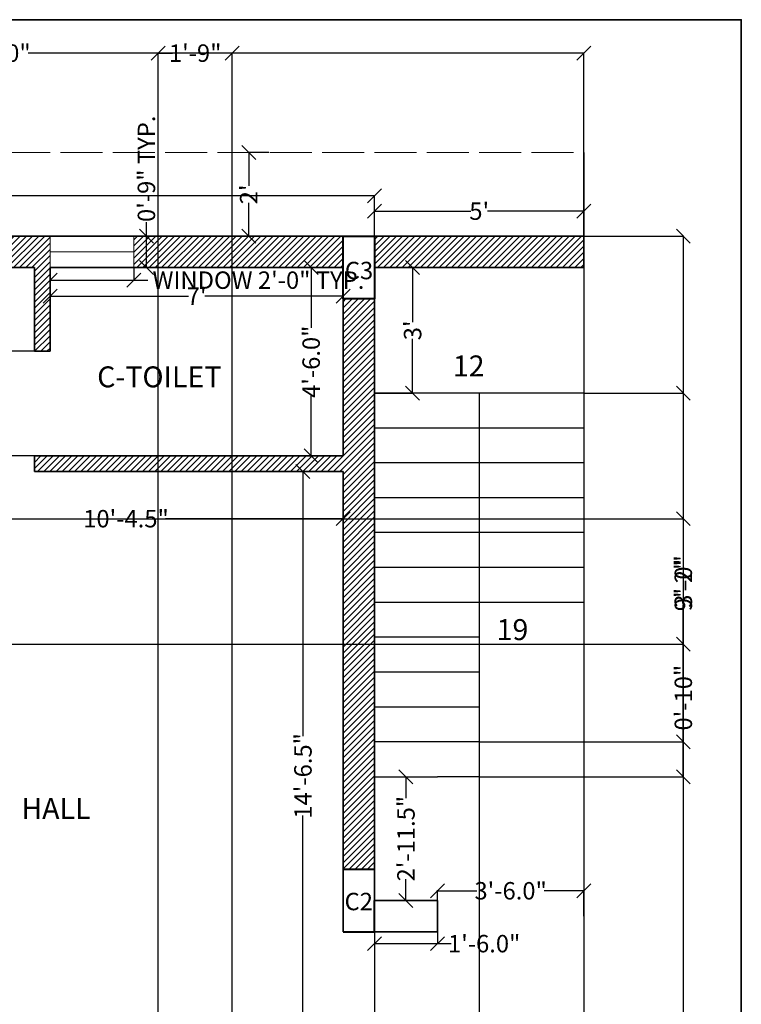
# Model space of a CAD drawing. Units: inches. Extents: x 72 to 538, y -43 to 598.
# Tile 4 of 4: x 331 to 538, y 316 to 598. Entities that reach past the tile are written whole.
import ezdxf

# ---------------------------------------------------------------- set-up
doc = ezdxf.new("R2010")
doc.units = ezdxf.units.IN
doc.header["$MEASUREMENT"] = 0
doc.linetypes.add('ACAD_ISO02W100', pattern=[15, 12, -3])
for name, color, linetype, lineweight in [('A-ANNO-DIMS', 2, 'Continuous', 18), ('A-ANNO-TEXT', 6, 'Continuous', 18), ('A-ANNO-TTLB', 7, 'Continuous', 35), ('A-AREA-IDEN', 7, 'Continuous', 25), ('A-COLS', 6, 'Continuous', 40), ('A-FLOR-STRS', 6, 'Continuous', 25), ('A-GLAZ', 4, 'Continuous', 18), ('A-WALL', 7, 'Continuous', 35), ('C-PROP', 3, 'ACAD_ISO02W100', 18), ('C-SITE', 7, 'Continuous', 25)]:
    doc.layers.add(name, color=color, linetype=linetype, lineweight=lineweight)
doc.layers.add('A-WALL-PATT', color=30, linetype='Continuous', lineweight=13, true_color=0xf26722)
doc.styles.get("Standard").update_dxf_attribs({"font": 'arial.ttf'})
doc.dimstyles.get("Standard").update_dxf_attribs({"dimtxt": 5, "dimasz": 4, "dimexe": 0.18, "dimexo": 0.0625, "dimgap": 0.09, "dimtad": 0, "dimdec": 1, "dimzin": 0, "dimdsep": 46, "dimlunit": 3, "dimtxsty": 'Standard', "dimblk": 'OBLIQUE', "dimcen": 0.09, "dimadec": 0, "dimazin": 0, "dimtfac": 1, "dimtdec": 1, "dimtofl": 0, "dimtmove": 0, "dimatfit": 3, "dimfxl": 1, "dimtolj": 1, "dimtzin": 0, "dimarcsym": 0})

# ---------------------------------------------------------------- blocks, each defined once
blk = doc.blocks.new('_Oblique')
at = {"color": 0, "linetype": 'ByBlock', "lineweight": -2}
blk.add_line((-0.5, -0.5), (0.5, 0.5), dxfattribs=at)
blk = doc.blocks.new('*D4')
at = {"layer": 'A-ANNO-DIMS', "color": 0, "lineweight": -2, "transparency": 16777216}
for p, q in [((423.57, 527.12), (414.27, 527.12)), ((414.45, 527.12), (414.45, 509.87)), ((414.45, 473.12), (414.45, 490.37)), ((423.57, 473.12), (414.27, 473.12))]:
    blk.add_line(p, q, dxfattribs=at)
at = {"layer": 'Defpoints', "color": 0, "transparency": 16777216}
for p in [(423.63, 527.12), (414.45, 473.12), (423.63, 473.12)]:
    blk.add_point(p, dxfattribs=at)
at = {"layer": 'A-ANNO-DIMS', "color": 0, "lineweight": -2, "transparency": 16777216, "xscale": 4, "yscale": 4, "zscale": 4}
for p, rotation in [((414.45, 527.12), 90), ((414.45, 473.12), 270)]:
    blk.add_blockref('_Oblique', p, dxfattribs=dict(at, rotation=rotation))
at = {"layer": 'A-ANNO-DIMS', "color": 0, "transparency": 16777216, "insert": (414.45, 500.12), "char_height": 5, "attachment_point": 5, "rotation": 90}
blk.add_mtext('\\A1;4\'-6.0"', dxfattribs=at)
blk = doc.blocks.new('*D5')
at = {"layer": 'A-ANNO-DIMS', "color": 0, "lineweight": -2, "transparency": 16777216}
for p, q in [((339.63, 518.18), (339.63, 519.11)), ((339.63, 518.93), (379.26, 518.93)), ((423.63, 518.93), (384, 518.93)), ((423.63, 518.18), (423.63, 519.11))]:
    blk.add_line(p, q, dxfattribs=at)
at = {"layer": 'Defpoints', "color": 0, "transparency": 16777216}
for p in [(339.63, 518.93), (339.63, 518.12), (423.63, 518.12)]:
    blk.add_point(p, dxfattribs=at)
at = {"layer": 'A-ANNO-DIMS', "color": 0, "lineweight": -2, "transparency": 16777216, "xscale": 4, "yscale": 4, "zscale": 4, "rotation": 180}
blk.add_blockref('_Oblique', (339.63, 518.93), dxfattribs=at)
at = {"layer": 'A-ANNO-DIMS', "color": 0, "lineweight": -2, "transparency": 16777216, "xscale": 4, "yscale": 4, "zscale": 4}
blk.add_blockref('_Oblique', (423.63, 518.93), dxfattribs=at)
at = {"layer": 'A-ANNO-DIMS', "color": 0, "transparency": 16777216, "insert": (381.63, 518.93), "char_height": 5, "attachment_point": 5}
blk.add_mtext("\\A1;7'", dxfattribs=at)
blk = doc.blocks.new('*D26')
at = {"layer": 'A-ANNO-DIMS', "color": 0, "lineweight": -2, "transparency": 16777216}
for p, q in [((299.13, 455.18), (299.13, 455.3)), ((299.13, 455.12), (350.02, 455.12)), ((423.63, 455.12), (372.73, 455.12)), ((423.63, 455.18), (423.63, 455.3))]:
    blk.add_line(p, q, dxfattribs=at)
at = {"layer": 'Defpoints', "color": 0, "transparency": 16777216}
for p in [(299.13, 455.12), (423.63, 455.12), (423.63, 455.12)]:
    blk.add_point(p, dxfattribs=at)
at = {"layer": 'A-ANNO-DIMS', "color": 0, "lineweight": -2, "transparency": 16777216, "xscale": 4, "yscale": 4, "zscale": 4, "rotation": 180}
blk.add_blockref('_Oblique', (299.13, 455.12), dxfattribs=at)
at = {"layer": 'A-ANNO-DIMS', "color": 0, "lineweight": -2, "transparency": 16777216, "xscale": 4, "yscale": 4, "zscale": 4}
blk.add_blockref('_Oblique', (423.63, 455.12), dxfattribs=at)
at = {"layer": 'A-ANNO-DIMS', "color": 0, "transparency": 16777216, "insert": (361.38, 455.12), "char_height": 5, "attachment_point": 5}
blk.add_mtext('\\A1;10\'-4.5"', dxfattribs=at)
blk = doc.blocks.new('*D27')
at = {"layer": 'A-ANNO-DIMS', "color": 0, "lineweight": -2, "transparency": 16777216}
for p, q in [((423.57, 468.62), (411.92, 468.62)), ((412.1, 468.62), (412.1, 392.73)), ((412.1, 294.12), (412.1, 370.01)), ((423.57, 294.12), (411.92, 294.12))]:
    blk.add_line(p, q, dxfattribs=at)
at = {"layer": 'Defpoints', "color": 0, "transparency": 16777216}
for p in [(423.63, 468.62), (412.1, 294.12), (423.63, 294.12)]:
    blk.add_point(p, dxfattribs=at)
at = {"layer": 'A-ANNO-DIMS', "color": 0, "lineweight": -2, "transparency": 16777216, "xscale": 4, "yscale": 4, "zscale": 4}
for p, rotation in [((412.1, 468.62), 90), ((412.1, 294.12), 270)]:
    blk.add_blockref('_Oblique', p, dxfattribs=dict(at, rotation=rotation))
at = {"layer": 'A-ANNO-DIMS', "color": 0, "transparency": 16777216, "insert": (412.1, 381.37), "char_height": 5, "attachment_point": 5, "rotation": 90}
blk.add_mtext('\\A1;14\'-6.5"', dxfattribs=at)
blk = doc.blocks.new('*D28')
at = {"layer": 'A-ANNO-DIMS', "color": 0, "lineweight": -2, "transparency": 16777216}
for p, q in [((432.63, 536.18), (432.63, 543.49)), ((432.63, 543.31), (460.24, 543.31)), ((492.63, 543.31), (465.02, 543.31)), ((492.63, 536.18), (492.63, 543.49))]:
    blk.add_line(p, q, dxfattribs=at)
at = {"layer": 'Defpoints', "color": 0, "transparency": 16777216}
for p in [(492.63, 543.31), (432.63, 536.12), (492.63, 536.12)]:
    blk.add_point(p, dxfattribs=at)
at = {"layer": 'A-ANNO-DIMS', "color": 0, "lineweight": -2, "transparency": 16777216, "xscale": 4, "yscale": 4, "zscale": 4, "rotation": 180}
blk.add_blockref('_Oblique', (432.63, 543.31), dxfattribs=at)
at = {"layer": 'A-ANNO-DIMS', "color": 0, "lineweight": -2, "transparency": 16777216, "xscale": 4, "yscale": 4, "zscale": 4}
blk.add_blockref('_Oblique', (492.63, 543.31), dxfattribs=at)
at = {"layer": 'A-ANNO-DIMS', "color": 0, "transparency": 16777216, "insert": (462.63, 543.31), "char_height": 5, "attachment_point": 5}
blk.add_mtext("\\A1;5'", dxfattribs=at)
blk = doc.blocks.new('*D29')
at = {"layer": 'A-ANNO-DIMS', "color": 0, "lineweight": -2, "transparency": 16777216}
for p, q in [((432.69, 527.12), (443.72, 527.12)), ((443.54, 527.12), (443.54, 511.51)), ((443.54, 491.12), (443.54, 506.73)), ((432.69, 491.12), (443.72, 491.12))]:
    blk.add_line(p, q, dxfattribs=at)
at = {"layer": 'Defpoints', "color": 0, "transparency": 16777216}
for p in [(432.63, 527.12), (432.63, 491.12), (443.54, 491.12)]:
    blk.add_point(p, dxfattribs=at)
at = {"layer": 'A-ANNO-DIMS', "color": 0, "lineweight": -2, "transparency": 16777216, "xscale": 4, "yscale": 4, "zscale": 4}
for p, rotation in [((443.54, 527.12), 90), ((443.54, 491.12), 270)]:
    blk.add_blockref('_Oblique', p, dxfattribs=dict(at, rotation=rotation))
at = {"layer": 'A-ANNO-DIMS', "color": 0, "transparency": 16777216, "insert": (443.54, 509.12), "char_height": 5, "attachment_point": 5, "rotation": 90}
blk.add_mtext("\\A1;3'", dxfattribs=at)
blk = doc.blocks.new('*D30')
at = {"layer": 'A-ANNO-DIMS', "color": 0, "lineweight": -2, "transparency": 16777216}
for p, q in [((441.63, 381.12), (441.63, 375)), ((441.69, 381.12), (441.81, 381.12)), ((441.63, 345.62), (441.63, 351.74)), ((441.69, 345.62), (441.81, 345.62))]:
    blk.add_line(p, q, dxfattribs=at)
at = {"layer": 'Defpoints', "color": 0, "transparency": 16777216}
for p in [(441.63, 381.12), (441.63, 381.12), (441.63, 345.62)]:
    blk.add_point(p, dxfattribs=at)
at = {"layer": 'A-ANNO-DIMS', "color": 0, "lineweight": -2, "transparency": 16777216, "xscale": 4, "yscale": 4, "zscale": 4}
for p, rotation in [((441.63, 381.12), 90), ((441.63, 345.62), 270)]:
    blk.add_blockref('_Oblique', p, dxfattribs=dict(at, rotation=rotation))
at = {"layer": 'A-ANNO-DIMS', "color": 0, "transparency": 16777216, "insert": (441.63, 363.37), "char_height": 5, "attachment_point": 5, "rotation": 90}
blk.add_mtext('\\A1;2\'-11.5"', dxfattribs=at)
blk = doc.blocks.new('*D31')
at = {"layer": 'A-ANNO-DIMS', "color": 0, "lineweight": -2, "transparency": 16777216}
for p, q in [((432.63, 336.56), (432.63, 333.08)), ((450.63, 336.56), (450.63, 333.08)), ((432.63, 333.26), (450.63, 333.26)), ((450.63, 333.26), (454.63, 333.26))]:
    blk.add_line(p, q, dxfattribs=at)
at = {"layer": 'Defpoints', "color": 0, "transparency": 16777216}
for p in [(432.63, 336.62), (450.63, 336.62), (450.63, 333.26)]:
    blk.add_point(p, dxfattribs=at)
at = {"layer": 'A-ANNO-DIMS', "color": 0, "lineweight": -2, "transparency": 16777216, "xscale": 4, "yscale": 4, "zscale": 4, "rotation": 180}
blk.add_blockref('_Oblique', (432.63, 333.26), dxfattribs=at)
at = {"layer": 'A-ANNO-DIMS', "color": 0, "lineweight": -2, "transparency": 16777216, "xscale": 4, "yscale": 4, "zscale": 4}
blk.add_blockref('_Oblique', (450.63, 333.26), dxfattribs=at)
at = {"layer": 'A-ANNO-DIMS', "color": 0, "transparency": 16777216, "insert": (464.04, 333.26), "char_height": 5, "attachment_point": 5}
blk.add_mtext('\\A1;1\'-6.0"', dxfattribs=at)
blk = doc.blocks.new('*D32')
at = {"layer": 'A-ANNO-DIMS', "color": 0, "lineweight": -2, "transparency": 16777216}
for p, q in [((450.63, 341.18), (450.63, 348.6)), ((450.63, 348.42), (461.98, 348.42)), ((492.63, 348.42), (481.28, 348.42)), ((492.63, 341.18), (492.63, 348.6))]:
    blk.add_line(p, q, dxfattribs=at)
at = {"layer": 'Defpoints', "color": 0, "transparency": 16777216}
for p in [(492.63, 348.42), (450.63, 341.12), (492.63, 341.12)]:
    blk.add_point(p, dxfattribs=at)
at = {"layer": 'A-ANNO-DIMS', "color": 0, "lineweight": -2, "transparency": 16777216, "xscale": 4, "yscale": 4, "zscale": 4, "rotation": 180}
blk.add_blockref('_Oblique', (450.63, 348.42), dxfattribs=at)
at = {"layer": 'A-ANNO-DIMS', "color": 0, "lineweight": -2, "transparency": 16777216, "xscale": 4, "yscale": 4, "zscale": 4}
blk.add_blockref('_Oblique', (492.63, 348.42), dxfattribs=at)
at = {"layer": 'A-ANNO-DIMS', "color": 0, "transparency": 16777216, "insert": (471.63, 348.42), "char_height": 5, "attachment_point": 5}
blk.add_mtext('\\A1;3\'-6.0"', dxfattribs=at)
blk = doc.blocks.new('*D37')
at = {"layer": 'A-ANNO-DIMS', "color": 0, "lineweight": -2, "transparency": 16777216}
for p, q in [((156.63, 536.18), (156.63, 547.9)), ((432.63, 536.18), (432.63, 547.9)), ((156.63, 547.72), (290.25, 547.72)), ((432.63, 547.72), (299, 547.72))]:
    blk.add_line(p, q, dxfattribs=at)
at = {"layer": 'Defpoints', "color": 0, "transparency": 16777216}
for p in [(432.63, 547.72), (156.63, 536.12), (432.63, 536.12)]:
    blk.add_point(p, dxfattribs=at)
at = {"layer": 'A-ANNO-DIMS', "color": 0, "lineweight": -2, "transparency": 16777216, "xscale": 4, "yscale": 4, "zscale": 4, "rotation": 180}
blk.add_blockref('_Oblique', (156.63, 547.72), dxfattribs=at)
at = {"layer": 'A-ANNO-DIMS', "color": 0, "lineweight": -2, "transparency": 16777216, "xscale": 4, "yscale": 4, "zscale": 4}
blk.add_blockref('_Oblique', (432.63, 547.72), dxfattribs=at)
at = {"layer": 'A-ANNO-DIMS', "color": 0, "transparency": 16777216, "insert": (294.63, 547.72), "char_height": 5, "attachment_point": 5}
blk.add_mtext("\\A1;23'", dxfattribs=at)
blk = doc.blocks.new('*D38')
at = {"layer": 'A-ANNO-DIMS', "color": 0, "lineweight": -2, "transparency": 16777216}
for p, q in [((402.33, 560.12), (396.37, 560.12)), ((396.55, 560.12), (396.55, 550.55)), ((396.55, 536.12), (396.55, 545.69)), ((402.33, 536.12), (396.37, 536.12))]:
    blk.add_line(p, q, dxfattribs=at)
at = {"layer": 'Defpoints', "color": 0, "transparency": 16777216}
for p in [(402.39, 560.12), (396.55, 536.12), (402.39, 536.12)]:
    blk.add_point(p, dxfattribs=at)
at = {"layer": 'A-ANNO-DIMS', "color": 0, "lineweight": -2, "transparency": 16777216, "xscale": 4, "yscale": 4, "zscale": 4}
for p, rotation in [((396.55, 560.12), 90), ((396.55, 536.12), 270)]:
    blk.add_blockref('_Oblique', p, dxfattribs=dict(at, rotation=rotation))
at = {"layer": 'A-ANNO-DIMS', "color": 0, "transparency": 16777216, "insert": (396.55, 548.12), "char_height": 5, "attachment_point": 5, "rotation": 90}
blk.add_mtext("\\A1;2'", dxfattribs=at)
blk = doc.blocks.new('COL-9X18')
for p, q in [((0, 18), (9, 18)), ((0, 0), (0, 18)), ((9, 18), (9, 0)), ((9, 0), (0, 0))]:
    blk.add_line(p, q)
blk = doc.blocks.new('WIN-24')
for p, q in [((0, 0), (0, 9)), ((24, 0), (24, 9)), ((0, 4.5), (24, 4.5))]:
    blk.add_line(p, q)
blk = doc.blocks.new('*D50')
at = {"layer": 'A-ANNO-DIMS', "color": 0, "lineweight": -2, "transparency": 16777216}
for p, q in [((339.63, 527.06), (339.63, 523.34)), ((363.63, 527.06), (363.63, 523.34)), ((339.63, 523.52), (363.63, 523.52)), ((363.63, 523.52), (367.63, 523.52))]:
    blk.add_line(p, q, dxfattribs=at)
at = {"layer": 'Defpoints', "color": 0, "transparency": 16777216}
for p in [(339.63, 527.12), (363.63, 527.12), (363.63, 523.52)]:
    blk.add_point(p, dxfattribs=at)
at = {"layer": 'A-ANNO-DIMS', "color": 0, "lineweight": -2, "transparency": 16777216, "xscale": 4, "yscale": 4, "zscale": 4, "rotation": 180}
blk.add_blockref('_Oblique', (339.63, 523.52), dxfattribs=at)
at = {"layer": 'A-ANNO-DIMS', "color": 0, "lineweight": -2, "transparency": 16777216, "xscale": 4, "yscale": 4, "zscale": 4}
blk.add_blockref('_Oblique', (363.63, 523.52), dxfattribs=at)
at = {"layer": 'A-ANNO-DIMS', "color": 0, "transparency": 16777216, "insert": (399.35, 523.52), "char_height": 5, "attachment_point": 5}
blk.add_mtext('\\A1;WINDOW 2\'-0" TYP.', dxfattribs=at)
blk = doc.blocks.new('*D51')
at = {"layer": 'A-ANNO-DIMS', "color": 0, "lineweight": -2, "transparency": 16777216}
for p, q in [((367.23, 536.12), (367.23, 540.12)), ((363.69, 536.12), (367.41, 536.12)), ((367.23, 527.12), (367.23, 536.12)), ((363.69, 527.12), (367.41, 527.12))]:
    blk.add_line(p, q, dxfattribs=at)
at = {"layer": 'Defpoints', "color": 0, "transparency": 16777216}
for p in [(363.63, 536.12), (367.23, 536.12), (363.63, 527.12)]:
    blk.add_point(p, dxfattribs=at)
at = {"layer": 'A-ANNO-DIMS', "color": 0, "lineweight": -2, "transparency": 16777216, "xscale": 4, "yscale": 4, "zscale": 4}
for p, rotation in [((367.23, 536.12), 90), ((367.23, 527.12), 270)]:
    blk.add_blockref('_Oblique', p, dxfattribs=dict(at, rotation=rotation))
at = {"layer": 'A-ANNO-DIMS', "color": 0, "transparency": 16777216, "insert": (367.23, 555.45), "char_height": 5, "attachment_point": 5, "rotation": 90}
blk.add_mtext('\\A1;0\'-9" TYP.', dxfattribs=at)
blk = doc.blocks.new('*D52')
at = {"layer": 'A-ANNO-DIMS', "color": 0, "lineweight": -2, "transparency": 16777216}
for p, q in [((156.63, 536.18), (156.63, 588.8)), ((156.63, 588.62), (315.91, 588.62)), ((492.63, 588.62), (333.35, 588.62)), ((492.63, 536.18), (492.63, 588.8))]:
    blk.add_line(p, q, dxfattribs=at)
at = {"layer": 'Defpoints', "color": 0, "transparency": 16777216}
for p in [(492.63, 588.62), (156.63, 536.12), (492.63, 536.12)]:
    blk.add_point(p, dxfattribs=at)
at = {"layer": 'A-ANNO-DIMS', "color": 0, "lineweight": -2, "transparency": 16777216, "xscale": 4, "yscale": 4, "zscale": 4, "rotation": 180}
blk.add_blockref('_Oblique', (156.63, 588.62), dxfattribs=at)
at = {"layer": 'A-ANNO-DIMS', "color": 0, "lineweight": -2, "transparency": 16777216, "xscale": 4, "yscale": 4, "zscale": 4}
blk.add_blockref('_Oblique', (492.63, 588.62), dxfattribs=at)
at = {"layer": 'A-ANNO-DIMS', "color": 0, "transparency": 16777216, "insert": (324.63, 588.62), "char_height": 5, "attachment_point": 5}
blk.add_mtext('\\A1;28\'-0"', dxfattribs=at)
blk = doc.blocks.new('*D53')
at = {"layer": 'A-ANNO-DIMS', "color": 0, "lineweight": -2, "transparency": 16777216}
for p, q in [((492.69, 536.12), (521.31, 536.12)), ((521.13, 536.12), (521.13, 295.9)), ((521.13, 38.12), (521.13, 278.34)), ((492.69, 38.12), (521.31, 38.12))]:
    blk.add_line(p, q, dxfattribs=at)
at = {"layer": 'Defpoints', "color": 0, "transparency": 16777216}
for p in [(492.63, 536.12), (521.13, 536.12), (492.63, 38.12)]:
    blk.add_point(p, dxfattribs=at)
at = {"layer": 'A-ANNO-DIMS', "color": 0, "lineweight": -2, "transparency": 16777216, "xscale": 4, "yscale": 4, "zscale": 4}
for p, rotation in [((521.13, 536.12), 90), ((521.13, 38.12), 270)]:
    blk.add_blockref('_Oblique', p, dxfattribs=dict(at, rotation=rotation))
at = {"layer": 'A-ANNO-DIMS', "color": 0, "transparency": 16777216, "insert": (521.13, 287.12), "char_height": 5, "attachment_point": 5, "rotation": 90}
blk.add_mtext('\\A1;41\'-6"', dxfattribs=at)
blk = doc.blocks.new('*D54')
at = {"layer": 'A-ANNO-DIMS', "color": 0, "lineweight": -2, "transparency": 16777216}
for p, q in [((432.63, 381.06), (432.63, -35.94)), ((462.63, 381.06), (462.63, -35.94)), ((432.63, -35.76), (440.85, -35.76)), ((462.63, -35.76), (454.41, -35.76))]:
    blk.add_line(p, q, dxfattribs=at)
at = {"layer": 'Defpoints', "color": 0, "transparency": 16777216}
for p in [(432.63, 381.12), (462.63, 381.12), (462.63, -35.76)]:
    blk.add_point(p, dxfattribs=at)
at = {"layer": 'A-ANNO-DIMS', "color": 0, "lineweight": -2, "transparency": 16777216, "xscale": 4, "yscale": 4, "zscale": 4, "rotation": 180}
blk.add_blockref('_Oblique', (432.63, -35.76), dxfattribs=at)
at = {"layer": 'A-ANNO-DIMS', "color": 0, "lineweight": -2, "transparency": 16777216, "xscale": 4, "yscale": 4, "zscale": 4}
blk.add_blockref('_Oblique', (462.63, -35.76), dxfattribs=at)
at = {"layer": 'A-ANNO-DIMS', "color": 0, "transparency": 16777216, "insert": (447.63, -35.76), "char_height": 5, "attachment_point": 5}
blk.add_mtext('\\A1;2\'-6"', dxfattribs=at)
blk = doc.blocks.new('*D55')
at = {"layer": 'A-ANNO-DIMS', "color": 0, "lineweight": -2, "transparency": 16777216}
for p, q in [((521.13, 391.12), (521.13, 395.12)), ((462.69, 391.12), (521.31, 391.12)), ((521.13, 381.12), (521.13, 391.12)), ((462.69, 381.12), (521.31, 381.12))]:
    blk.add_line(p, q, dxfattribs=at)
at = {"layer": 'Defpoints', "color": 0, "transparency": 16777216}
for p in [(462.63, 391.12), (521.13, 391.12), (462.63, 381.12)]:
    blk.add_point(p, dxfattribs=at)
at = {"layer": 'A-ANNO-DIMS', "color": 0, "lineweight": -2, "transparency": 16777216, "xscale": 4, "yscale": 4, "zscale": 4}
for p, rotation in [((521.13, 391.12), 90), ((521.13, 381.12), 270)]:
    blk.add_blockref('_Oblique', p, dxfattribs=dict(at, rotation=rotation))
at = {"layer": 'A-ANNO-DIMS', "color": 0, "transparency": 16777216, "insert": (521.13, 403.8), "char_height": 5, "attachment_point": 5, "rotation": 90}
blk.add_mtext('\\A1;0\'-10"', dxfattribs=at)
blk = doc.blocks.new('*D56')
at = {"layer": 'A-ANNO-DIMS', "color": 0, "lineweight": -2, "transparency": 16777216}
for p, q in [((492.69, 491.12), (521.31, 491.12)), ((521.13, 491.12), (521.13, 442.86)), ((521.13, 381.12), (521.13, 429.38)), ((462.69, 381.12), (521.31, 381.12))]:
    blk.add_line(p, q, dxfattribs=at)
at = {"layer": 'Defpoints', "color": 0, "transparency": 16777216}
for p in [(492.63, 491.12), (521.13, 491.12), (462.63, 381.12)]:
    blk.add_point(p, dxfattribs=at)
at = {"layer": 'A-ANNO-DIMS', "color": 0, "lineweight": -2, "transparency": 16777216, "xscale": 4, "yscale": 4, "zscale": 4}
for p, rotation in [((521.13, 491.12), 90), ((521.13, 381.12), 270)]:
    blk.add_blockref('_Oblique', p, dxfattribs=dict(at, rotation=rotation))
at = {"layer": 'A-ANNO-DIMS', "color": 0, "transparency": 16777216, "insert": (521.13, 436.12), "char_height": 5, "attachment_point": 5, "rotation": 90}
blk.add_mtext('\\A1;9\'-2"', dxfattribs=at)
blk = doc.blocks.new('*D60')
at = {"layer": 'A-ANNO-DIMS', "color": 0, "lineweight": -2, "transparency": 16777216}
for p, q in [((370.61, 89.18), (370.61, 588.8)), ((370.61, 588.62), (374.71, 588.62)), ((391.82, 588.62), (387.71, 588.62)), ((391.82, 89.18), (391.82, 588.8))]:
    blk.add_line(p, q, dxfattribs=at)
at = {"layer": 'Defpoints', "color": 0, "transparency": 16777216}
for p in [(391.82, 588.62), (370.61, 89.12), (391.82, 89.12)]:
    blk.add_point(p, dxfattribs=at)
at = {"layer": 'A-ANNO-DIMS', "color": 0, "lineweight": -2, "transparency": 16777216, "xscale": 4, "yscale": 4, "zscale": 4, "rotation": 180}
blk.add_blockref('_Oblique', (370.61, 588.62), dxfattribs=at)
at = {"layer": 'A-ANNO-DIMS', "color": 0, "lineweight": -2, "transparency": 16777216, "xscale": 4, "yscale": 4, "zscale": 4}
blk.add_blockref('_Oblique', (391.82, 588.62), dxfattribs=at)
at = {"layer": 'A-ANNO-DIMS', "color": 0, "transparency": 16777216, "insert": (381.21, 588.62), "char_height": 5, "attachment_point": 5}
blk.add_mtext('\\A1;1\'-9"', dxfattribs=at)
blk = doc.blocks.new('*D62')
at = {"layer": 'A-ANNO-DIMS', "color": 0, "lineweight": -2, "transparency": 16777216}
for p, q in [((339.57, 503.12), (103.95, 503.12)), ((104.13, 503.12), (104.13, 494.9)), ((104.13, 473.12), (104.13, 481.34)), ((339.57, 473.12), (103.95, 473.12))]:
    blk.add_line(p, q, dxfattribs=at)
at = {"layer": 'Defpoints', "color": 0, "transparency": 16777216}
for p in [(339.63, 503.12), (104.13, 473.12), (339.63, 473.12)]:
    blk.add_point(p, dxfattribs=at)
at = {"layer": 'A-ANNO-DIMS', "color": 0, "lineweight": -2, "transparency": 16777216, "xscale": 4, "yscale": 4, "zscale": 4}
for p, rotation in [((104.13, 503.12), 90), ((104.13, 473.12), 270)]:
    blk.add_blockref('_Oblique', p, dxfattribs=dict(at, rotation=rotation))
at = {"layer": 'A-ANNO-DIMS', "color": 0, "transparency": 16777216, "insert": (104.13, 488.12), "char_height": 5, "attachment_point": 5, "rotation": 90}
blk.add_mtext('\\A1;2\'-6"', dxfattribs=at)
blk = doc.blocks.new('*D63')
at = {"layer": 'A-ANNO-DIMS', "color": 0, "lineweight": -2, "transparency": 16777216}
for p, q in [((294.69, 455.12), (521.31, 455.12)), ((521.13, 455.12), (521.13, 443.85)), ((521.13, 419.12), (521.13, 430.39)), ((299.19, 419.12), (521.31, 419.12))]:
    blk.add_line(p, q, dxfattribs=at)
at = {"layer": 'Defpoints', "color": 0, "transparency": 16777216}
for p in [(294.63, 455.12), (299.13, 419.12), (521.13, 419.12)]:
    blk.add_point(p, dxfattribs=at)
at = {"layer": 'A-ANNO-DIMS', "color": 0, "lineweight": -2, "transparency": 16777216, "xscale": 4, "yscale": 4, "zscale": 4}
for p, rotation in [((521.13, 455.12), 90), ((521.13, 419.12), 270)]:
    blk.add_blockref('_Oblique', p, dxfattribs=dict(at, rotation=rotation))
at = {"layer": 'A-ANNO-DIMS', "color": 0, "transparency": 16777216, "insert": (521.13, 437.12), "char_height": 5, "attachment_point": 5, "rotation": 90}
blk.add_mtext('\\A1;3\'-0"', dxfattribs=at)

msp = doc.modelspace()

# ---------------------------------------------------------------- hatches: boundary and pattern name
at = {"layer": 'A-WALL-PATT'}
h = msp.add_hatch(dxfattribs=at)
h.set_pattern_fill('ANSI31', color=256, scale=10)
h.paths.add_polyline_path([(204.03, 536.12), (165.63, 536.12), (165.63, 527.12), (204.03, 527.12)])
h.paths.add_polyline_path([(165.63, 487.18), (165.63, 518.12), (156.63, 518.12), (156.63, 487.18)])
h.paths.add_polyline_path([(374.85, 253.74), (416.04, 253.74), (416.04, 266.11), (374.85, 266.11)], flags=9)
h.paths.add_polyline_path([(358.05, 165.41), (382.02, 165.41), (382.02, 177.78), (358.05, 177.78)], flags=9)
h.paths.add_polyline_path([(258.82, 340.82), (290.25, 340.82), (290.25, 353.18), (258.82, 353.18)], flags=9)
h.paths.add_polyline_path([(190.8, 385.39), (230.59, 385.39), (230.59, 397.75), (190.8, 397.75)], flags=9)
h.paths.add_polyline_path([(259.76, 122.35), (291.18, 122.35), (291.18, 134.72), (259.76, 134.72)], flags=9)
h.paths.add_polyline_path([(192.66, 147.9), (232.45, 147.9), (232.45, 160.26), (192.66, 160.26)], flags=9)
h.paths.add_polyline_path([(197.84, 250.21), (246.48, 250.21), (246.48, 262.58), (197.84, 262.58)], flags=9)
h.paths.add_polyline_path([(329.22, 365.75), (353.18, 365.75), (353.18, 378.11), (329.22, 378.11)], flags=9)
h.paths.add_polyline_path([(351.21, 489.41), (392.39, 489.41), (392.39, 501.77), (351.21, 501.77)], flags=9)
h.paths.add_polyline_path([(193.31, 469.76), (241.95, 469.76), (241.95, 482.12), (193.31, 482.12)], flags=9)
h.paths.add_polyline_path([(262.62, 413.67), (274.04, 413.67), (274.04, 423.97), (262.62, 423.97)], flags=9)
h.paths.add_polyline_path([(155.57, 341.76), (167, 341.76), (167, 352.06), (155.57, 352.06)], flags=9)
h.paths.add_polyline_path([(155.43, 129.83), (166.86, 129.83), (166.86, 140.14), (155.43, 140.14)], flags=9)
h.paths.add_polyline_path([(293.27, 137.19), (304.7, 137.19), (304.7, 147.49), (293.27, 147.49)], flags=9)
h.paths.add_polyline_path([(440.6, 145.74), (452.03, 145.74), (452.03, 156.04), (440.6, 156.04)], flags=9)
h.paths.add_polyline_path([(422.43, 340.03), (433.86, 340.03), (433.86, 350.33), (422.43, 350.33)], flags=9)
h.paths.add_polyline_path([(155.47, 520.54), (166.9, 520.54), (166.9, 530.84), (155.47, 530.84)], flags=9)
h.paths.add_polyline_path([(348.1, 449.93), (374.22, 449.93), (374.22, 460.24), (348.1, 460.24)], flags=9)
h.paths.add_polyline_path([(417.29, 368.09), (417.29, 394.21), (406.99, 394.21), (406.99, 368.09)], flags=9)
h.paths.add_polyline_path([(422.51, 520.96), (433.94, 520.96), (433.94, 531.26), (422.51, 531.26)], flags=9)
h.paths.add_polyline_path([(284.05, 526.61), (295.48, 526.61), (295.48, 536.92), (284.05, 536.92)], flags=9)
h = msp.add_hatch(dxfattribs=at)
h.set_pattern_fill('ANSI31', color=256, scale=10)
h.paths.add_polyline_path([(432.63, 468.62), (432.63, 518.12), (423.63, 518.12), (423.63, 473.12), (339.63, 473.12), (335.13, 473.12), (335.13, 468.62), (423.63, 468.62), (423.63, 354.62), (432.63, 354.62)])
h.paths.add_polyline_path([(450.63, 231.12), (450.63, 240.93), (441.63, 240.93), (441.63, 235.62), (357.63, 235.62), (353.13, 235.62), (353.13, 231.12), (441.63, 231.12)])
h.paths.add_polyline_path([(374.85, 253.74), (416.04, 253.74), (416.04, 266.11), (374.85, 266.11)], flags=9)
h.paths.add_polyline_path([(358.05, 165.41), (382.02, 165.41), (382.02, 177.78), (358.05, 177.78)], flags=9)
h.paths.add_polyline_path([(258.82, 340.82), (290.25, 340.82), (290.25, 353.18), (258.82, 353.18)], flags=9)
h.paths.add_polyline_path([(190.8, 385.39), (230.59, 385.39), (230.59, 397.75), (190.8, 397.75)], flags=9)
h.paths.add_polyline_path([(259.76, 122.35), (291.18, 122.35), (291.18, 134.72), (259.76, 134.72)], flags=9)
h.paths.add_polyline_path([(192.66, 147.9), (232.45, 147.9), (232.45, 160.26), (192.66, 160.26)], flags=9)
h.paths.add_polyline_path([(197.84, 250.21), (246.48, 250.21), (246.48, 262.58), (197.84, 262.58)], flags=9)
h.paths.add_polyline_path([(329.22, 365.75), (353.18, 365.75), (353.18, 378.11), (329.22, 378.11)], flags=9)
h.paths.add_polyline_path([(351.21, 489.41), (392.39, 489.41), (392.39, 501.77), (351.21, 501.77)], flags=25)
h.paths.add_polyline_path([(193.31, 469.76), (241.95, 469.76), (241.95, 482.12), (193.31, 482.12)], flags=9)
h.paths.add_polyline_path([(262.62, 413.67), (274.04, 413.67), (274.04, 423.97), (262.62, 423.97)], flags=9)
h.paths.add_polyline_path([(155.57, 341.76), (167, 341.76), (167, 352.06), (155.57, 352.06)], flags=9)
h.paths.add_polyline_path([(155.43, 129.83), (166.86, 129.83), (166.86, 140.14), (155.43, 140.14)], flags=9)
h.paths.add_polyline_path([(293.27, 137.19), (304.7, 137.19), (304.7, 147.49), (293.27, 147.49)], flags=9)
h.paths.add_polyline_path([(440.6, 145.74), (452.03, 145.74), (452.03, 156.04), (440.6, 156.04)], flags=9)
h.paths.add_polyline_path([(422.43, 340.03), (433.86, 340.03), (433.86, 350.33), (422.43, 350.33)], flags=9)
h.paths.add_polyline_path([(422.51, 520.96), (433.94, 520.96), (433.94, 531.26), (422.51, 531.26)], flags=9)
h.paths.add_polyline_path([(284.05, 526.61), (295.48, 526.61), (295.48, 536.92), (284.05, 536.92)], flags=9)
h.paths.add_polyline_path([(155.47, 520.54), (166.9, 520.54), (166.9, 530.84), (155.47, 530.84)], flags=9)
h = msp.add_hatch(dxfattribs=at)
h.set_pattern_fill('ANSI31', color=256, scale=10)
h.paths.add_polyline_path([(165.63, 427.18), (156.63, 427.18), (156.63, 414.62), (165.63, 414.62), (258.91, 414.62), (258.91, 419.12), (165.63, 419.12)])
h.paths.add_polyline_path([(165.63, 378.62), (156.63, 378.62), (156.63, 355.53), (165.63, 355.53)])
h.paths.add_polyline_path([(299.13, 378.12), (290.13, 378.12), (290.13, 373.62), (294.63, 373.62), (294.63, 318.12), (252.63, 318.12), (252.63, 373.62), (257.13, 373.62), (257.13, 378.12), (248.13, 378.12), (248.13, 318.12), (165.63, 318.12), (165.63, 337.53), (156.63, 337.53), (156.63, 294.2), (165.63, 294.2), (165.63, 313.62), (294.63, 313.62), (294.63, 289.62), (312.63, 289.62), (312.63, 235.62), (294.63, 235.62), (294.63, 231.12), (317.13, 231.12), (317.13, 289.62), (353.13, 289.62), (353.13, 265.62), (357.63, 265.62), (357.63, 289.62), (441.63, 289.62), (441.63, 264.93), (450.63, 264.93), (450.63, 294.12), (432.63, 294.12), (299.13, 294.12)])
h.paths.add_polyline_path([(299.13, 195.12), (165.63, 195.12), (165.63, 234.2), (156.63, 234.2), (156.63, 144.66), (165.63, 144.66), (165.63, 190.62), (299.13, 190.62)])
h.paths.add_polyline_path([(165.63, 126.66), (156.63, 126.66), (156.63, 80.12), (212.13, 80.12), (212.13, 89.12), (165.63, 89.12)])
h.paths.add_polyline_path([(310.61, 89.12), (299.13, 89.12), (299.13, 137.87), (294.63, 137.87), (294.63, 89.12), (252.63, 89.12), (252.63, 144.62), (257.13, 144.62), (257.13, 149.12), (248.13, 149.12), (248.13, 89.12), (248.13, 80.12), (310.61, 80.12)])
h.paths.add_polyline_path([(450.63, 142.12), (441.63, 142.12), (441.63, 89.12), (433.82, 89.12), (433.82, 80.12), (450.63, 80.12)])
h.paths.add_polyline_path([(450.63, 171.12), (446.13, 171.12), (441.63, 171.12), (441.63, 160.12), (450.63, 160.12)])
h.paths.add_polyline_path([(281.13, 536.12), (264.03, 536.12), (264.03, 527.12), (281.13, 527.12)])
h.paths.add_polyline_path([(339.63, 536.12), (299.13, 536.12), (299.13, 527.12), (335.13, 527.12), (335.13, 503.12), (339.63, 503.12), (339.63, 527.12)])
h.paths.add_polyline_path([(299.13, 527.12), (294.63, 527.12), (294.63, 455.12), (299.13, 455.12)])
h.paths.add_polyline_path([(492.63, 536.12), (432.63, 536.12), (432.63, 527.12), (492.63, 527.12)])
h.paths.add_polyline_path([(423.63, 536.12), (363.63, 536.12), (363.63, 527.12), (423.63, 527.12)])
h.paths.add_polyline_path([(299.13, 419.12), (276.91, 419.12), (276.91, 414.62), (299.13, 414.62)])

# ---------------------------------------------------------------- linework, layer by layer
at = {"layer": 'A-ANNO-TTLB'}
msp.add_lwpolyline([(72.29, 598.2), (537.75, 598.2), (537.75, -7.26), (72.29, -7.26)], close=True, dxfattribs=at)
at = {"layer": 'A-COLS'}
for p, q in [((423.63, 354.62), (432.63, 354.62)), ((432.63, 336.62), (432.63, 345.62)), ((423.63, 336.62), (432.63, 336.62))]:
    msp.add_line(p, q, dxfattribs=at)
at = {"layer": 'A-FLOR-STRS'}
for p, q in [((492.63, 491.12), (432.63, 491.12)), ((462.63, 491.12), (462.63, 381.12)), ((492.63, 481.12), (432.63, 481.12)), ((492.63, 471.12), (432.63, 471.12)), ((492.63, 461.12), (432.63, 461.12)), ((492.63, 451.12), (432.63, 451.12)), ((492.63, 441.12), (432.63, 441.12)), ((492.63, 431.12), (432.63, 431.12)), ((462.63, 421.12), (432.63, 421.12)), ((462.63, 411.12), (432.63, 411.12)), ((462.63, 401.12), (432.63, 401.12)), ((462.63, 391.12), (432.63, 391.12)), ((432.63, 381.12), (450.63, 381.12)), ((462.63, 381.12), (450.63, 381.12))]:
    msp.add_line(p, q, dxfattribs=at)
at = {"layer": 'A-WALL'}
for p, q in [((156.63, 536.12), (432.63, 536.12)), ((432.63, 536.12), (432.63, 336.62)), ((432.63, 536.12), (492.63, 536.12)), ((492.63, 536.12), (492.63, 527.12)), ((299.13, 527.12), (335.13, 527.12)), ((335.13, 527.12), (335.13, 503.12)), ((339.63, 527.12), (339.63, 503.12)), ((339.63, 527.12), (423.63, 527.12)), ((423.63, 527.12), (423.63, 473.12)), ((492.63, 527.12), (432.63, 527.12)), ((339.63, 503.12), (335.13, 503.12)), ((339.63, 473.12), (335.13, 473.12)), ((335.13, 473.12), (335.13, 468.62)), ((339.63, 473.12), (423.63, 473.12)), ((335.13, 468.62), (423.63, 468.62)), ((423.63, 468.62), (423.63, 336.62)), ((423.63, 336.62), (423.63, 468.62)), ((432.63, 468.62), (432.63, 336.62)), ((432.63, 345.62), (450.63, 345.62)), ((450.63, 345.62), (450.63, 336.62)), ((432.63, 336.62), (423.63, 336.62)), ((450.63, 336.62), (432.63, 336.62))]:
    msp.add_line(p, q, dxfattribs=at)
at = {"layer": 'C-PROP'}
msp.add_line((132.63, 560.12), (492.63, 560.12), dxfattribs=at)
at = {"layer": 'C-SITE'}
msp.add_line((492.63, 560.12), (492.63, -7.26), dxfattribs=at)

# ---------------------------------------------------------------- block references
at = {"layer": 'A-COLS'}
msp.add_blockref('COL-9X18', (423.63, 518.12), dxfattribs=at)
at = {"layer": 'A-GLAZ'}
msp.add_blockref('WIN-24', (339.63, 527.12), dxfattribs=at)

# ---------------------------------------------------------------- texts
at = {"layer": 'A-ANNO-TEXT', "attachment_point": 1}
for s, width, insert, char_height in [('C3', 12, (424.1, 528.78), 5), ('12', 78.4308, (455.07, 501.92), 6), ('19', 78.4308, (467.62, 426.31), 6), ('C2', 12, (424.03, 347.84), 5)]:
    msp.add_mtext_dynamic_manual_height_columns(s, width=width, gutter_width=1, heights=[0], dxfattribs=dict(at, insert=insert, char_height=char_height))
at = {"layer": 'A-AREA-IDEN', "char_height": 6, "attachment_point": 1}
for s, insert in [('C-TOILET', (353.12, 498.79)), ('HALL', (331.39, 375.02))]:
    msp.add_mtext_dynamic_manual_height_columns(s, width=78.4308, gutter_width=1, heights=[0], dxfattribs=dict(at, insert=insert))

# ---------------------------------------------------------------- dimensions: what is measured, and where the dimension line sits
at = {"layer": 'A-ANNO-DIMS'}
for base, p1, p2, override, picture, middle in [((492.63, 588.62), (156.63, 536.12), (492.63, 536.12), {"dimdec": 1, "dimlfac": 1, "dimrnd": 0, "dimzin": 1, "dimdsep": 46, "dimlunit": 4, "dimfrac": 2}, '*D52', (324.63, 588.62)), ((391.82, 588.62), (370.61, 89.12), (391.82, 89.12), {"dimdec": 1, "dimlfac": 1, "dimrnd": 0, "dimzin": 1, "dimdsep": 46, "dimlunit": 4, "dimfrac": 2}, '*D60', (381.21, 588.62)), ((432.63, 547.72), (156.63, 536.12), (432.63, 536.12), {"dimclrd": 0, "dimclre": 0, "dimclrt": 0}, '*D37', (294.63, 547.72)), ((492.63, 543.31), (432.63, 536.12), (492.63, 536.12), {"dimclrd": 0, "dimclre": 0, "dimclrt": 0}, '*D28', (462.63, 543.31)), ((339.63, 518.93), (423.63, 518.12), (339.63, 518.12), {"dimclrd": 0, "dimclre": 0, "dimclrt": 0}, '*D5', (381.63, 518.93)), ((423.63, 455.12), (299.13, 455.12), (423.63, 455.12), {"dimclrd": 0, "dimclre": 0, "dimclrt": 0}, '*D26', (361.38, 455.12)), ((462.63, -35.76), (432.63, 381.12), (462.63, 381.12), {"dimdec": 1, "dimlfac": 1, "dimrnd": 0, "dimzin": 1, "dimdsep": 46, "dimlunit": 4, "dimfrac": 2}, '*D54', (447.63, -35.76)), ((492.63, 348.42), (450.63, 341.12), (492.63, 341.12), {"dimclrd": 0, "dimclre": 0, "dimclrt": 0}, '*D32', (471.63, 348.42)), ((450.63, 333.26), (432.63, 336.62), (450.63, 336.62), {"dimclrd": 0, "dimclre": 0, "dimclrt": 0}, '*D31', (464.04, 333.26))]:
    dim = msp.add_linear_dim(base=base, p1=p1, p2=p2, dimstyle='Standard', override=override, dxfattribs=at)
    dim.commit()
    dim.dimension.update_dxf_attribs({"geometry": picture, "text_midpoint": middle})
dim = msp.add_linear_dim(base=(367.23, 536.12), p1=(363.63, 527.12), p2=(363.63, 536.12), angle=90, text='<> TYP.', dimstyle='Standard', override={"dimdec": 1, "dimlfac": 1, "dimrnd": 0, "dimzin": 1, "dimdsep": 46, "dimlunit": 4, "dimfrac": 2}, dxfattribs=at)
dim.commit()
dim.dimension.update_dxf_attribs({"geometry": '*D51', "text_midpoint": (367.23, 555.45)})
for base, p1, p2, override, picture, middle in [((396.55, 536.12), (402.39, 560.12), (402.39, 536.12), {"dimclrd": 0, "dimclre": 0, "dimclrt": 0}, '*D38', (396.55, 548.12)), ((521.13, 536.12), (492.63, 38.12), (492.63, 536.12), {"dimdec": 1, "dimlfac": 1, "dimrnd": 0, "dimzin": 1, "dimdsep": 46, "dimlunit": 4, "dimfrac": 2}, '*D53', (521.13, 287.12)), ((414.45, 473.12), (423.63, 527.12), (423.63, 473.12), {"dimclrd": 0, "dimclre": 0, "dimclrt": 0}, '*D4', (414.45, 500.12)), ((443.54, 491.12), (432.63, 527.12), (432.63, 491.12), {"dimclrd": 0, "dimclre": 0, "dimclrt": 0}, '*D29', (443.54, 509.12)), ((104.13, 473.12), (339.63, 503.12), (339.63, 473.12), {"dimdec": 1, "dimlfac": 1, "dimrnd": 0, "dimzin": 1, "dimdsep": 46, "dimlunit": 4, "dimfrac": 2}, '*D62', (104.13, 488.12)), ((521.13, 491.12), (462.63, 381.12), (492.63, 491.12), {"dimdec": 1, "dimlfac": 1, "dimrnd": 0, "dimzin": 1, "dimdsep": 46, "dimlunit": 4, "dimfrac": 2}, '*D56', (521.13, 436.12)), ((412.1, 294.12), (423.63, 468.62), (423.63, 294.12), {"dimclrd": 0, "dimclre": 0, "dimclrt": 0}, '*D27', (412.1, 381.37)), ((521.13, 419.12), (294.63, 455.12), (299.13, 419.12), {"dimdec": 1, "dimlfac": 1, "dimrnd": 0, "dimzin": 1, "dimdsep": 46, "dimlunit": 4, "dimfrac": 2}, '*D63', (521.13, 437.12)), ((521.13, 391.12), (462.63, 381.12), (462.63, 391.12), {"dimdec": 1, "dimlfac": 1, "dimrnd": 0, "dimzin": 1, "dimdsep": 46, "dimlunit": 4, "dimfrac": 2}, '*D55', (521.13, 403.8)), ((441.63, 381.12), (441.63, 345.62), (441.63, 381.12), {"dimclrd": 0, "dimclre": 0, "dimclrt": 0}, '*D30', (441.63, 363.37))]:
    dim = msp.add_linear_dim(base=base, p1=p1, p2=p2, angle=90, dimstyle='Standard', override=override, dxfattribs=at)
    dim.commit()
    dim.dimension.update_dxf_attribs({"geometry": picture, "text_midpoint": middle})
dim = msp.add_linear_dim(base=(363.63, 523.52), p1=(339.63, 527.12), p2=(363.63, 527.12), text='WINDOW <> TYP.', dimstyle='Standard', override={"dimdec": 1, "dimlfac": 1, "dimrnd": 0, "dimzin": 1, "dimdsep": 46, "dimlunit": 4, "dimfrac": 2}, dxfattribs=at)
dim.commit()
dim.dimension.update_dxf_attribs({"geometry": '*D50', "text_midpoint": (399.35, 523.52)})

doc.saveas('drawing.dxf')
